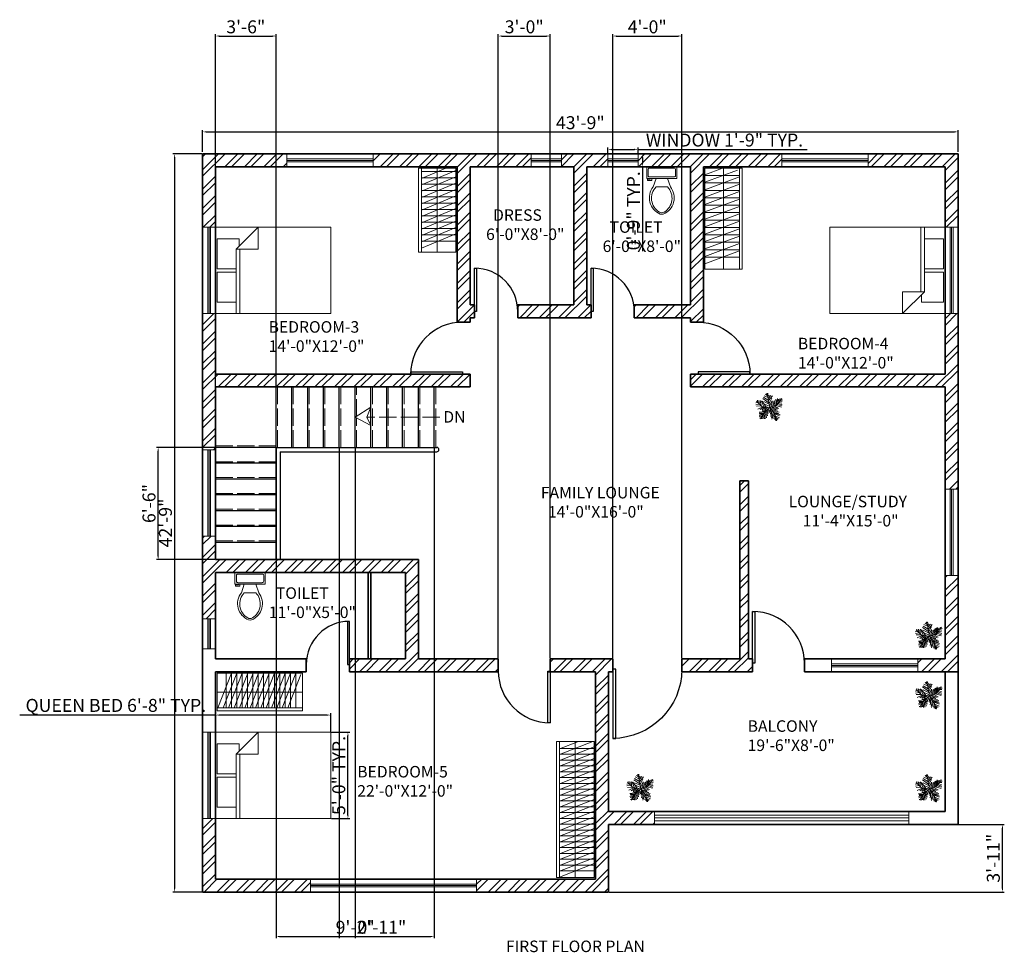
# Model space of a CAD drawing. Units: inches. Extents: x 451 to 1761, y 2292 to 3014.
# Tile 3 of 3: x 1077 to 1761, y 2303 to 2952. Entities that reach past the tile are written whole.
import ezdxf

# ---------------------------------------------------------------- set-up
doc = ezdxf.new("R2010")
doc.units = ezdxf.units.IN
doc.linetypes.add('ACAD_ISO02W100', pattern=[15, 12, -3])
for name, color, linetype, lineweight in [('A-ANNO-DIMS', 2, 'Continuous', 18), ('A-ANNO-PATH', 7, 'ACAD_ISO02W100', 18), ('A-ANNO-SYMB', 7, 'Continuous', 18), ('A-ANNO-TEXT', 7, 'Continuous', 25), ('A-AREA-IDEN', 7, 'Continuous', 18), ('A-DOOR', 4, 'Continuous', 25), ('A-FLOR-CASE', 9, 'Continuous', 18), ('A-FLOR-CASE-PATT', 252, 'Continuous', 13), ('A-FLOR-FIXT', 9, 'Continuous', 18), ('A-FLOR-RAIL', 244, 'Continuous', 18), ('A-FLOR-STRS', 7, 'Continuous', 25), ('A-FLOR-STRS-HIDN', 8, 'ACAD_ISO02W100', 13), ('A-FURN', 8, 'Continuous', 18), ('A-GLAZ', 244, 'Continuous', 18), ('A-WALL', 7, 'Continuous', 35), ('A-WALL-PATT', 252, 'Continuous', 13), ('L-PLNT', 3, 'Continuous', 18)]:
    doc.layers.add(name, color=color, linetype=linetype, lineweight=lineweight)
doc.styles.get("Standard").update_dxf_attribs({"font": 'arial.ttf'})
doc.dimstyles.new('ISO-25', dxfattribs={"dimtxt": 9, "dimasz": 2.5, "dimexe": 1.25, "dimexo": 0.625, "dimtad": 1, "dimlunit": 3, "dimtxsty": 'Standard', "dimcen": 2.5, "dimadec": 0, "dimazin": 0, "dimtfac": 1, "dimtmove": 0, "dimatfit": 3, "dimfxl": 1, "dimarcsym": 0})

# ---------------------------------------------------------------- blocks, each defined once
blk = doc.blocks.new('*U14')
for p, q in [((-40, 0), (-40, 6)), ((0, 0), (0, 6))]:
    blk.add_line(p, q)
blk.add_lwpolyline([(0, 0), (0, -40), (-1.75, -40), (-1.75, 0)], close=True)
blk.add_arc((0, 0), 40, 180, 270)
blk = doc.blocks.new('*U15')
for p, q in [((0, 0), (0, -6)), ((-40, 0), (-40, -6))]:
    blk.add_line(p, q)
blk.add_lwpolyline([(0, 0), (0, 40), (-1.75, 40), (-1.75, 0)], close=True)
blk.add_arc((0, 0), 40, 90, 180)
blk = doc.blocks.new('*U16')
for p, q in [((0, 0), (0, -6)), ((40, 0), (40, -6))]:
    blk.add_line(p, q)
blk.add_lwpolyline([(0, 0), (0, 40), (1.75, 40), (1.75, 0)], close=True)
blk.add_arc((0, 0), 40, 0, 90)
blk = doc.blocks.new('Bed - Queen')
for p, q in [((0, -80.00003), (0, 0)), ((0, 0), (59.99999, 0)), ((59.99999, 0), (59.99999, -80.00003)), ((7.99999, -1.2), (28.79998, -1.2)), ((7.99999, -14.4), (7.99999, -1.2)), ((28.79998, -1.2), (28.79998, -14.4)), ((31.19999, -1.2), (51.99999, -1.2)), ((31.19999, -14.4), (31.19999, -1.2)), ((51.99999, -1.2), (51.99999, -16.4)), ((0, -14.4), (44.8, -14.4)), ((44.8, -16.8), (0, -16.8)), ((59.99999, -29.6), (44.8, -14.4)), ((44.8, -14.4), (44.8, -29.6)), ((51.99999, -16.4), (46.79936, -16.4)), ((44.8, -29.6), (59.99999, -29.6)), ((59.99999, -80.00003), (0, -80.00003))]:
    blk.add_line(p, q)
blk = doc.blocks.new('*U10')
for p, q in [((9.5, -6), (9.5, -2)), ((-10, -8.5), (-8, -8.5)), ((-10, -9.5), (-10, -8.5)), ((-7, -9.5), (-10, -9.5)), ((-8, -8.5), (-8, -8)), ((-7, -8), (-7, -9.5)), ((-4, -8), (-6, -14)), ((4, -8), (6, -14)), ((4, -14), (-4, -14))]:
    blk.add_line(p, q)
blk.add_lwpolyline([(10.5, -8), (10.5, 0), (-10.5, 0), (-10.5, -8)], close=True)
for points in [[(-9.5, -2), (-9.5, -6)], [(8.5, -1), (-8.5, -1)], [(-8.5, -7), (8.5, -7)]]:
    blk.add_lwpolyline(points)
for centre, radius, start, end in [((-8.62, -1.88), 0.884, 81.8699, 188.1301), ((-8.62, -6.12), 0.884, 171.8699, 278.1301), ((8.62, -1.88), 0.884, 351.8699, 98.1301), ((8.62, -6.12), 0.884, 261.8699, 8.1301), ((3.52, -21.58), 12.17, 141.46911, 247.97143), ((4.2, -21.82), 11.33, 136.36773, 238.94682), ((-3.52, -21.58), 12.17, 292.02843, 38.53071), ((-4.2, -21.82), 11.33, 301.05301, 43.63209), ((0, -27.88), 4, 245.73182, 294.26817), ((0, -29), 4, 254.86053, 285.13947)]:
    blk.add_arc(centre, radius, start, end)
blk = doc.blocks.new('*U12')
for p, q in [((-5.114, 28.097), (-24.676, 40.636)), ((-7.288, 39.707), (-21.778, 46.673)), ((-8.737, 47.138), (-17.069, 52.711)), ((-10.186, 53.64), (-13.084, 55.962)), ((0, 0), (-10.5, 57)), ((-9.099, 51.782), (-6.563, 55.962)), ((-7.65, 43.423), (-2.578, 49.46)), ((-5.839, 35.992), (4.667, 48.067)), ((-5.114, 27.632), (10.463, 46.673)), ((-47.498, 19.737), (-55.83, 18.344)), ((-40.615, 13.7), (-55.105, 10.913)), ((-31.5, 4.5), (-52.5, 25.5)), ((-33.37, 6.269), (-52.207, 5.34)), ((-48.585, 21.131), (-49.309, 29.026)), ((-28.299, 3.483), (-47.86, -5.805)), ((-43.513, 28.561), (-42.427, 15.558)), ((-38.442, 26.239), (-34.819, 7.663)), ((-21.416, 3.018), (-38.079, -8.128)), ((-35.544, 28.097), (-24.314, 3.947)), ((0, 0), (-31.5, 4.5)), ((-14.533, 2.09), (-30.834, 25.31)), ((-15.982, 2.09), (-30.11, -9.521)), ((-3.665, 19.273), (-27.574, 35.527)), ((-24.314, 23.917), (-2.941, 13.7)), ((0, 0), (-22.5, -19.5)), ((-6.563, 1.161), (-21.416, -8.128)), ((-20.691, 13.7), (-1.129, 4.876)), ((-2.941, 16.486), (8.652, 37.85)), ((-1.129, 6.734), (9.014, 26.704)), ((0, 0), (27, 9)), ((0, 0), (18, -22.5)), ((3.942, 1.625), (11.187, 24.381)), ((6.478, 1.625), (26.04, -8.592)), ((10.101, 3.483), (17.708, 26.239)), ((11.187, 3.483), (30.749, -5.805)), ((16.259, 5.805), (23.142, 31.348)), ((18.07, 5.805), (35.096, -3.483)), ((22.055, 7.198), (27.489, 32.277)), ((24.229, 7.663), (46.688, 1.625)), ((27, 9), (48, 36)), ((27.127, 9.056), (31.112, 35.992)), ((29.662, 12.307), (48.137, 6.269)), ((31.836, 30.883), (32.561, 16.486)), ((33.285, 16.486), (48.862, 10.913)), ((35.096, 32.741), (37.27, 22.524)), ((36.183, 19.737), (48.137, 17.88)), ((38.719, 34.134), (41.979, 28.561)), ((40.53, 25.775), (48.862, 24.846)), ((43.791, 29.954), (51.036, 30.883)), ((44.153, 36.456), (45.239, 32.741)), ((-17.431, -15.094), (-42.789, -18.809)), ((-28.299, -29.026), (-42.789, -31.348)), ((-24.314, -21.596), (-42.427, -22.06)), ((-30.834, -34.135), (-42.427, -35.528)), ((-26.849, -26.24), (-40.253, -25.775)), ((-22.5, -19.5), (-37.5, -45)), ((-32.646, -36.921), (-31.921, -44.352)), ((-15.257, -12.772), (-30.11, -12.772)), ((-29.023, -30.884), (-27.936, -43.887)), ((-25.038, -23.918), (-22.865, -45.281)), ((-20.691, -18.345), (-17.793, -44.352)), ((-6.563, -5.805), (-19.967, -9.985)), ((-17.069, -15.094), (-12.721, -40.172)), ((-13.446, -11.378), (-8.737, -32.741)), ((-9.461, -8.592), (-6.201, -23.453)), ((-4.752, -3.483), (-3.665, -14.629)), ((2.493, -3.019), (-1.491, -20.202)), ((1.769, -2.555), (24.229, -9.521)), ((5.029, -6.27), (2.131, -25.775)), ((9.014, -11.378), (3.58, -35.992)), ((14.085, -16.951), (6.478, -40.172)), ((7.565, -9.056), (32.198, -14.629)), ((18.07, -22.524), (8.289, -45.745)), ((12.274, -15.094), (36.907, -18.809)), ((20.244, -30.419), (15.897, -44.816)), ((16.259, -19.738), (36.183, -22.989)), ((18, -22.5), (27, -52.5)), ((18.433, -22.524), (40.53, -29.026)), ((19.157, -25.311), (38.719, -33.206)), ((22.78, -37.85), (19.519, -48.532)), ((21.331, -32.741), (39.081, -40.636)), ((22.78, -38.314), (34.372, -44.816)), ((-34.457, -39.708), (-40.978, -42.494)), ((24.591, -45.745), (23.142, -50.854)), ((24.591, -43.423), (30.749, -47.603)), ((26.764, -49.925), (28.213, -50.854))]:
    blk.add_line(p, q)
blk = doc.blocks.new('*D19')
at = {"layer": 'A-ANNO-DIMS', "color": 0, "lineweight": -2, "transparency": 16777216}
for p, q in [((1203.82, 2859.74), (1203.82, 2874.82)), ((1728.82, 2859.74), (1728.82, 2874.82)), ((1206.32, 2873.57), (1726.32, 2873.57))]:
    blk.add_line(p, q, dxfattribs=at)
at = {"layer": 'A-ANNO-DIMS', "color": 0, "transparency": 16777216}
for points in [[(1206.32, 2873.99), (1206.32, 2873.15), (1203.82, 2873.57)], [(1726.32, 2873.99), (1726.32, 2873.15), (1728.82, 2873.57)]]:
    blk.add_solid(points, dxfattribs=at)
at = {"layer": 'Defpoints', "color": 0, "transparency": 16777216}
for p in [(1728.82, 2873.57), (1203.82, 2859.11), (1728.82, 2859.11)]:
    blk.add_point(p, dxfattribs=at)
at = {"layer": 'A-ANNO-DIMS', "color": 0, "transparency": 16777216, "insert": (1466.32, 2878.79), "char_height": 9, "attachment_point": 5}
blk.add_mtext('43\'-9"', dxfattribs=at)
blk = doc.blocks.new('*D20')
at = {"layer": 'A-ANNO-DIMS', "color": 0, "lineweight": -2, "transparency": 16777216}
for p, q in [((1203.19, 2858.28), (1183.1, 2858.28)), ((1184.35, 2855.78), (1184.35, 2347.78)), ((1203.19, 2345.28), (1183.1, 2345.28))]:
    blk.add_line(p, q, dxfattribs=at)
at = {"layer": 'A-ANNO-DIMS', "color": 0, "transparency": 16777216}
for points in [[(1183.94, 2855.78), (1184.77, 2855.78), (1184.35, 2858.28)], [(1183.94, 2347.78), (1184.77, 2347.78), (1184.35, 2345.28)]]:
    blk.add_solid(points, dxfattribs=at)
at = {"layer": 'Defpoints', "color": 0, "transparency": 16777216}
for p in [(1203.82, 2858.28), (1184.35, 2345.28), (1203.82, 2345.28)]:
    blk.add_point(p, dxfattribs=at)
at = {"layer": 'A-ANNO-DIMS', "color": 0, "transparency": 16777216, "insert": (1179.13, 2601.78), "char_height": 9, "attachment_point": 5, "rotation": 90}
blk.add_mtext('42\'-9"', dxfattribs=at)
blk = doc.blocks.new('WIN-60IN')
for p, q in [((0, 5.5), (60, 5.5)), ((0, 4.5), (60, 4.5)), ((0, 3.5), (60, 3.5))]:
    blk.add_line(p, q)
blk.add_lwpolyline([(0, 0), (0, 9), (60, 9), (60, 0)], close=True)
blk = doc.blocks.new('WIN-21IN')
for p, q in [((3.5, 0), (3.5, 21)), ((4.5, 0), (4.5, 21)), ((5.5, 0), (5.5, 21))]:
    blk.add_line(p, q)
blk.add_lwpolyline([(0, 0), (0, 21), (9, 21), (9, 0)], close=True)
blk = doc.blocks.new('*D26')
at = {"layer": 'A-ANNO-DIMS', "color": 0, "lineweight": -2, "transparency": 16777216}
for p, q in [((1212.82, 2468.28), (1076.68, 2468.28)), ((1212.82, 2456.9), (1212.82, 2469.53)), ((1290.32, 2468.28), (1215.32, 2468.28)), ((1292.82, 2456.9), (1292.82, 2469.53))]:
    blk.add_line(p, q, dxfattribs=at)
at = {"layer": 'A-ANNO-DIMS', "color": 0, "transparency": 16777216}
for points in [[(1215.32, 2468.69), (1215.32, 2467.86), (1212.82, 2468.28)], [(1290.32, 2468.69), (1290.32, 2467.86), (1292.82, 2468.28)]]:
    blk.add_solid(points, dxfattribs=at)
at = {"layer": 'Defpoints', "color": 0, "transparency": 16777216}
for p in [(1212.82, 2468.28), (1212.82, 2456.28), (1292.82, 2456.28)]:
    blk.add_point(p, dxfattribs=at)
at = {"layer": 'A-ANNO-DIMS', "color": 0, "transparency": 16777216, "insert": (1143.5, 2473.83), "char_height": 9, "attachment_point": 5}
blk.add_mtext('QUEEN BED 6\'-8" TYP.', dxfattribs=at)
blk = doc.blocks.new('*D27')
at = {"layer": 'A-ANNO-DIMS', "color": 0, "lineweight": -2, "transparency": 16777216}
for p, q in [((1293.44, 2456.28), (1306.07, 2456.28)), ((1304.82, 2398.78), (1304.82, 2453.78)), ((1293.44, 2396.28), (1306.07, 2396.28))]:
    blk.add_line(p, q, dxfattribs=at)
at = {"layer": 'A-ANNO-DIMS', "color": 0, "transparency": 16777216}
for points in [[(1304.4, 2453.78), (1305.23, 2453.78), (1304.82, 2456.28)], [(1304.4, 2398.78), (1305.23, 2398.78), (1304.82, 2396.28)]]:
    blk.add_solid(points, dxfattribs=at)
at = {"layer": 'Defpoints', "color": 0, "transparency": 16777216}
for p in [(1292.82, 2456.28), (1304.82, 2456.28), (1292.82, 2396.28)]:
    blk.add_point(p, dxfattribs=at)
at = {"layer": 'A-ANNO-DIMS', "color": 0, "transparency": 16777216, "insert": (1299.6, 2426.28), "char_height": 9, "attachment_point": 5, "rotation": 90}
blk.add_mtext('5\'-0" TYP.', dxfattribs=at)
blk = doc.blocks.new('*D28')
at = {"layer": 'A-ANNO-DIMS', "color": 0, "lineweight": -2, "transparency": 16777216}
for p, q in [((1485.42, 2858.9), (1485.42, 2862.68)), ((1487.92, 2861.43), (1503.92, 2861.43)), ((1506.42, 2858.9), (1506.42, 2862.68)), ((1506.42, 2861.43), (1624.06, 2861.43))]:
    blk.add_line(p, q, dxfattribs=at)
at = {"layer": 'A-ANNO-DIMS', "color": 0, "transparency": 16777216}
for points in [[(1487.92, 2861.84), (1487.92, 2861.01), (1485.42, 2861.43)], [(1503.92, 2861.84), (1503.92, 2861.01), (1506.42, 2861.43)]]:
    blk.add_solid(points, dxfattribs=at)
at = {"layer": 'Defpoints', "color": 0, "transparency": 16777216}
for p in [(1506.42, 2861.43), (1485.42, 2858.28), (1506.42, 2858.28)]:
    blk.add_point(p, dxfattribs=at)
at = {"layer": 'A-ANNO-DIMS', "color": 0, "transparency": 16777216, "insert": (1566.49, 2866.71), "char_height": 9, "attachment_point": 5}
blk.add_mtext('WINDOW 1\'-9" TYP.', dxfattribs=at)
blk = doc.blocks.new('*D29')
at = {"layer": 'A-ANNO-DIMS', "color": 0, "lineweight": -2, "transparency": 16777216}
for p, q in [((1507.05, 2858.28), (1510.82, 2858.28)), ((1509.57, 2855.78), (1509.57, 2851.78)), ((1507.05, 2849.28), (1510.82, 2849.28)), ((1509.57, 2849.28), (1509.57, 2790.67))]:
    blk.add_line(p, q, dxfattribs=at)
at = {"layer": 'A-ANNO-DIMS', "color": 0, "transparency": 16777216}
for points in [[(1509.16, 2855.78), (1509.99, 2855.78), (1509.57, 2858.28)], [(1509.16, 2851.78), (1509.99, 2851.78), (1509.57, 2849.28)]]:
    blk.add_solid(points, dxfattribs=at)
at = {"layer": 'Defpoints', "color": 0, "transparency": 16777216}
for p in [(1506.42, 2858.28), (1506.42, 2849.28), (1509.57, 2849.28)]:
    blk.add_point(p, dxfattribs=at)
at = {"layer": 'A-ANNO-DIMS', "color": 0, "transparency": 16777216, "insert": (1504.35, 2818.72), "char_height": 9, "attachment_point": 5, "rotation": 90}
blk.add_mtext('0\'-9" TYP.', dxfattribs=at)
blk = doc.blocks.new('*D41')
at = {"layer": 'A-ANNO-DIMS', "color": 0, "lineweight": -2, "transparency": 16777216}
for p, q in [((1254.82, 2653.65), (1254.82, 2313.13)), ((1364.82, 2653.65), (1364.82, 2313.13)), ((1257.32, 2314.38), (1362.32, 2314.38))]:
    blk.add_line(p, q, dxfattribs=at)
at = {"layer": 'A-ANNO-DIMS', "color": 0, "transparency": 16777216}
for points in [[(1257.32, 2314.79), (1257.32, 2313.96), (1254.82, 2314.38)], [(1362.32, 2314.79), (1362.32, 2313.96), (1364.82, 2314.38)]]:
    blk.add_solid(points, dxfattribs=at)
at = {"layer": 'Defpoints', "color": 0, "transparency": 16777216}
for p in [(1254.82, 2654.28), (1364.82, 2654.28), (1364.82, 2314.38)]:
    blk.add_point(p, dxfattribs=at)
at = {"layer": 'A-ANNO-DIMS', "color": 0, "transparency": 16777216, "insert": (1309.82, 2319.6), "char_height": 9, "attachment_point": 5}
blk.add_mtext('9\'-2"', dxfattribs=at)
blk = doc.blocks.new('*D42')
at = {"layer": 'A-ANNO-DIMS', "color": 0, "lineweight": -2, "transparency": 16777216}
for p, q in [((1212.19, 2654.28), (1171.67, 2654.28)), ((1172.92, 2578.78), (1172.92, 2651.78)), ((1212.19, 2576.28), (1171.67, 2576.28))]:
    blk.add_line(p, q, dxfattribs=at)
at = {"layer": 'A-ANNO-DIMS', "color": 0, "transparency": 16777216}
for points in [[(1172.5, 2651.78), (1173.33, 2651.78), (1172.92, 2654.28)], [(1172.5, 2578.78), (1173.33, 2578.78), (1172.92, 2576.28)]]:
    blk.add_solid(points, dxfattribs=at)
at = {"layer": 'Defpoints', "color": 0, "transparency": 16777216}
for p in [(1172.92, 2654.28), (1212.82, 2654.28), (1212.82, 2576.28)]:
    blk.add_point(p, dxfattribs=at)
at = {"layer": 'A-ANNO-DIMS', "color": 0, "transparency": 16777216, "insert": (1167.7, 2615.28), "char_height": 9, "attachment_point": 5, "rotation": 90}
blk.add_mtext('6\'-6"', dxfattribs=at)
blk = doc.blocks.new('*D43')
at = {"layer": 'A-ANNO-DIMS', "color": 0, "lineweight": -2, "transparency": 16777216}
for p, q in [((1212.82, 2576.9), (1212.82, 2941.43)), ((1215.32, 2940.18), (1252.32, 2940.18)), ((1254.82, 2576.9), (1254.82, 2941.43))]:
    blk.add_line(p, q, dxfattribs=at)
at = {"layer": 'A-ANNO-DIMS', "color": 0, "transparency": 16777216}
for points in [[(1215.32, 2940.59), (1215.32, 2939.76), (1212.82, 2940.18)], [(1252.32, 2940.59), (1252.32, 2939.76), (1254.82, 2940.18)]]:
    blk.add_solid(points, dxfattribs=at)
at = {"layer": 'Defpoints', "color": 0, "transparency": 16777216}
for p in [(1254.82, 2940.18), (1212.82, 2576.28), (1254.82, 2576.28)]:
    blk.add_point(p, dxfattribs=at)
at = {"layer": 'A-ANNO-DIMS', "color": 0, "transparency": 16777216, "insert": (1233.82, 2945.4), "char_height": 9, "attachment_point": 5}
blk.add_mtext('3\'-6"', dxfattribs=at)
blk = doc.blocks.new('*D44')
at = {"layer": 'A-ANNO-DIMS', "color": 0, "lineweight": -2, "transparency": 16777216}
for p, q in [((1298.82, 2653.65), (1298.82, 2313.13)), ((1309.82, 2653.65), (1309.82, 2313.13)), ((1301.32, 2314.38), (1307.32, 2314.38)), ((1309.82, 2314.38), (1344.48, 2314.38))]:
    blk.add_line(p, q, dxfattribs=at)
at = {"layer": 'A-ANNO-DIMS', "color": 0, "transparency": 16777216}
for points in [[(1301.32, 2314.79), (1301.32, 2313.96), (1298.82, 2314.38)], [(1307.32, 2314.79), (1307.32, 2313.96), (1309.82, 2314.38)]]:
    blk.add_solid(points, dxfattribs=at)
at = {"layer": 'Defpoints', "color": 0, "transparency": 16777216}
for p in [(1298.82, 2654.28), (1309.82, 2654.28), (1309.82, 2314.38)]:
    blk.add_point(p, dxfattribs=at)
at = {"layer": 'A-ANNO-DIMS', "color": 0, "transparency": 16777216, "insert": (1328.4, 2319.6), "char_height": 9, "attachment_point": 5}
blk.add_mtext('0\'-11"', dxfattribs=at)
blk = doc.blocks.new('*D45')
at = {"layer": 'A-ANNO-DIMS', "color": 0, "lineweight": -2, "transparency": 16777216}
for p, q in [((1486.44, 2392.24), (1760.97, 2392.24)), ((1759.72, 2347.78), (1759.72, 2389.74)), ((1486.44, 2345.28), (1760.97, 2345.28))]:
    blk.add_line(p, q, dxfattribs=at)
at = {"layer": 'A-ANNO-DIMS', "color": 0, "transparency": 16777216}
for points in [[(1759.3, 2389.74), (1760.13, 2389.74), (1759.72, 2392.24)], [(1759.3, 2347.78), (1760.13, 2347.78), (1759.72, 2345.28)]]:
    blk.add_solid(points, dxfattribs=at)
at = {"layer": 'Defpoints', "color": 0, "transparency": 16777216}
for p in [(1485.82, 2392.24), (1759.72, 2392.24), (1485.82, 2345.28)]:
    blk.add_point(p, dxfattribs=at)
at = {"layer": 'A-ANNO-DIMS', "color": 0, "transparency": 16777216, "insert": (1754.49, 2368.76), "char_height": 9, "attachment_point": 5, "rotation": 90}
blk.add_mtext('3\'-11"', dxfattribs=at)
blk = doc.blocks.new('*D46')
at = {"layer": 'A-ANNO-DIMS', "color": 0, "lineweight": -2, "transparency": 16777216}
for p, q in [((1409.32, 2507.9), (1409.32, 2941.43)), ((1411.82, 2940.18), (1442.82, 2940.18)), ((1445.32, 2507.9), (1445.32, 2941.43))]:
    blk.add_line(p, q, dxfattribs=at)
at = {"layer": 'A-ANNO-DIMS', "color": 0, "transparency": 16777216}
for points in [[(1411.82, 2940.59), (1411.82, 2939.76), (1409.32, 2940.18)], [(1442.82, 2940.59), (1442.82, 2939.76), (1445.32, 2940.18)]]:
    blk.add_solid(points, dxfattribs=at)
at = {"layer": 'Defpoints', "color": 0, "transparency": 16777216}
for p in [(1445.32, 2940.18), (1409.32, 2507.28), (1445.32, 2507.28)]:
    blk.add_point(p, dxfattribs=at)
at = {"layer": 'A-ANNO-DIMS', "color": 0, "transparency": 16777216, "insert": (1427.32, 2945.4), "char_height": 9, "attachment_point": 5}
blk.add_mtext('3\'-0"', dxfattribs=at)
blk = doc.blocks.new('*D47')
at = {"layer": 'A-ANNO-DIMS', "color": 0, "lineweight": -2, "transparency": 16777216}
for p, q in [((1488.82, 2507.9), (1488.82, 2941.43)), ((1491.32, 2940.18), (1534.32, 2940.18)), ((1536.82, 2507.9), (1536.82, 2941.43))]:
    blk.add_line(p, q, dxfattribs=at)
at = {"layer": 'A-ANNO-DIMS', "color": 0, "transparency": 16777216}
for points in [[(1491.32, 2940.59), (1491.32, 2939.76), (1488.82, 2940.18)], [(1534.32, 2940.59), (1534.32, 2939.76), (1536.82, 2940.18)]]:
    blk.add_solid(points, dxfattribs=at)
at = {"layer": 'Defpoints', "color": 0, "transparency": 16777216}
for p in [(1536.82, 2940.18), (1488.82, 2507.28), (1536.82, 2507.28)]:
    blk.add_point(p, dxfattribs=at)
at = {"layer": 'A-ANNO-DIMS', "color": 0, "transparency": 16777216, "insert": (1512.82, 2945.4), "char_height": 9, "attachment_point": 5}
blk.add_mtext('4\'-0"', dxfattribs=at)

msp = doc.modelspace()

# ---------------------------------------------------------------- hatches: boundary and pattern name
at = {"layer": 'A-FLOR-CASE-PATT'}
h = msp.add_hatch(dxfattribs=at)
h.set_pattern_fill('ANSI31', color=256, scale=1.281376, angle=-22.43333, style=0)
h.paths.add_polyline_path([(1355.816, 2789.86), (1379.816, 2799.834), (1379.816, 2848.297), (1369.164, 2848.276), (1355.816, 2842.729)])
h = msp.add_hatch(dxfattribs=at)
h.set_pattern_fill('ANSI31', color=256, scale=1.387624, angle=-45, style=0)
h.paths.add_polyline_path([(1355.816, 2794.266), (1379.816, 2794.266), (1379.816, 2847.135), (1355.816, 2847.135)])
h = msp.add_hatch(dxfattribs=at)
h.set_pattern_fill('ANSI31', color=256, scale=1.520558, angle=-24.6033, style=0)
h.paths.add_polyline_path([(1552.816, 2778.252), (1576.816, 2787.176), (1576.816, 2843.834), (1574.909, 2848.276), (1561.057, 2848.276), (1552.816, 2845.212)])
h = msp.add_hatch(dxfattribs=at)
h.set_pattern_fill('ANSI31', color=256, scale=1.622274, angle=135, style=0)
h.paths.add_polyline_path([(1552.816, 2783.403), (1576.816, 2783.403), (1576.816, 2845.212), (1552.816, 2845.212)])
h = msp.add_hatch(dxfattribs=at)
h.set_pattern_fill('ANSI31', color=256, scale=1.0926, angle=23.3975, style=0)
h.paths.add_polyline_path([(1213.816, 2473.276), (1266.051, 2473.276), (1273.315, 2491.62), (1271.824, 2497.276), (1223.319, 2497.276)])
h = msp.add_hatch(dxfattribs=at)
h.set_pattern_fill('ANSI31', color=256, scale=1.175145, angle=45, style=0)
h.paths.add_polyline_path([(1217.547, 2473.276), (1269.782, 2473.276), (1269.782, 2497.276), (1217.547, 2497.276)])
h = msp.add_hatch(dxfattribs=at)
h.set_pattern_fill('ANSI31', color=256, scale=1.188375, angle=-23.51425, style=0)
h.paths.add_polyline_path([(1451.816, 2355.276), (1475.816, 2364.723), (1475.816, 2449.875), (1465.831, 2450), (1455.529, 2450), (1451.816, 2448.538)])
h = msp.add_hatch(dxfattribs=at)
h.set_pattern_fill('ANSI31', color=256, scale=1.277126, angle=-45, style=0)
h.paths.add_polyline_path([(1451.816, 2359.331), (1475.816, 2359.331), (1475.816, 2448.538), (1451.816, 2448.538)])
at = {"layer": 'A-WALL-PATT'}
h = msp.add_hatch(dxfattribs=at)
h.set_pattern_fill('ANSI32', color=256)
h.paths.add_polyline_path([(1473.81, 2753.276), (1470.816, 2753.276), (1470.816, 2849.276), (1485.423, 2849.276), (1485.423, 2858.276), (1453.123, 2858.276), (1453.123, 2849.276), (1461.816, 2849.276), (1461.816, 2753.276), (1422.483, 2753.276, -0.0376447), (1422.822, 2748.777), (1422.822, 2744.276), (1473.81, 2744.276), (1473.81, 2748.777)])
h.paths.add_polyline_path([(1551.816, 2849.276), (1606.235, 2849.276), (1606.235, 2858.276), (1506.423, 2858.276), (1506.423, 2849.276), (1542.816, 2849.276), (1542.816, 2753.276), (1503.816, 2753.276), (1503.816, 2744.276), (1542.816, 2744.276), (1542.816, 2741.276), (1548.216, 2741.276), (1551.816, 2741.276)])
h.paths.add_polyline_path([(1392.816, 2753.276), (1389.816, 2753.276), (1389.816, 2849.276), (1432.123, 2849.276), (1432.123, 2858.276), (1380.816, 2858.276), (1322.316, 2858.276), (1322.316, 2849.276), (1380.816, 2849.276), (1380.816, 2741.276), (1389.816, 2741.276), (1389.816, 2744.276), (1392.816, 2744.276)])
h.paths.add_polyline_path([(1728.816, 2747.276), (1719.816, 2747.276), (1719.816, 2705.276), (1551.816, 2705.276), (1548.216, 2705.276), (1542.816, 2705.276), (1542.816, 2696.276), (1719.816, 2696.276), (1719.816, 2625.296), (1728.816, 2625.296)])
h.paths.add_polyline_path([(1212.816, 2849.276), (1262.316, 2849.276), (1262.316, 2858.276), (1203.816, 2858.276), (1203.816, 2807.276), (1212.816, 2807.276)])
h.paths.add_polyline_path([(1728.816, 2858.276), (1666.235, 2858.276), (1666.235, 2849.276), (1719.816, 2849.276), (1719.816, 2807.276), (1728.816, 2807.276)])
h.paths.add_polyline_path([(1353.816, 2576.276), (1212.816, 2576.276), (1212.816, 2592.62), (1203.816, 2592.62), (1203.816, 2535.234), (1212.816, 2535.234), (1212.816, 2567.276), (1344.816, 2567.276), (1344.816, 2507.276), (1305.816, 2507.276), (1305.816, 2503.377), (1305.816, 2498.276), (1409.316, 2498.276), (1409.316, 2507.276), (1353.816, 2507.276)])
h.paths.add_polyline_path([(1728.816, 2565.296), (1719.816, 2565.296), (1719.816, 2507.276), (1700.944, 2507.276), (1700.944, 2498.276), (1719.816, 2498.276), (1728.816, 2498.276)])
h.paths.add_polyline_path([(1583.073, 2631.034), (1577.073, 2631.034), (1577.073, 2507.276), (1536.816, 2507.276), (1536.816, 2498.276), (1586.073, 2498.276), (1586.073, 2507.276), (1583.073, 2507.276)])
h = msp.add_hatch(dxfattribs=at)
h.set_pattern_fill('ANSI32', color=256)
h.paths.add_polyline_path([(1389.816, 2705.276), (1384.416, 2705.276), (1348.416, 2705.276), (1212.816, 2705.276), (1212.816, 2747.276), (1203.816, 2747.276), (1203.816, 2652.62), (1212.816, 2652.62), (1212.816, 2696.276), (1389.816, 2696.276)])
h.paths.add_polyline_path([(1278.816, 2354.276), (1212.816, 2354.276), (1212.816, 2396.276), (1203.816, 2396.276), (1203.816, 2345.276), (1278.816, 2345.276)])
h = msp.add_hatch(dxfattribs=at)
h.set_pattern_fill('ANSI32', color=256)
h.paths.add_polyline_path([(1485.816, 2392.237), (1517.902, 2392.237), (1517.902, 2401.237), (1485.816, 2401.237), (1485.816, 2498.276), (1488.816, 2498.276), (1488.816, 2507.276), (1445.316, 2507.276), (1445.316, 2498.276), (1476.816, 2498.276), (1476.816, 2354.276), (1394.234, 2354.276), (1394.234, 2345.276), (1485.816, 2345.276)])

# ---------------------------------------------------------------- linework, layer by layer
at = {"layer": 'A-ANNO-PATH'}
msp.add_line((1368.565, 2675.276), (1317.944, 2675.276), dxfattribs=at)
at = {"layer": 'A-ANNO-SYMB'}
for p, q in [((1309.816, 2675.276), (1320.816, 2682.17)), ((1317.944, 2675.276), (1320.816, 2682.17)), ((1309.816, 2675.276), (1320.816, 2669.469)), ((1320.816, 2669.469), (1317.944, 2675.276))]:
    msp.add_line(p, q, dxfattribs=at)
at = {"layer": 'A-FLOR-CASE'}
for p, q in [((1353.816, 2848.276), (1379.816, 2848.276)), ((1353.816, 2848.276), (1353.816, 2789.86)), ((1355.816, 2848.276), (1355.816, 2789.86)), ((1366.816, 2848.276), (1366.816, 2789.86)), ((1379.816, 2848.276), (1379.816, 2789.86)), ((1552.816, 2848.276), (1552.816, 2778.252)), ((1552.816, 2848.276), (1578.816, 2848.276)), ((1565.816, 2848.276), (1565.816, 2778.252)), ((1576.816, 2848.276), (1576.816, 2778.252)), ((1578.816, 2848.276), (1578.816, 2778.252)), ((1379.816, 2789.86), (1353.816, 2789.86)), ((1552.816, 2778.252), (1578.816, 2778.252)), ((1213.816, 2497.276), (1273.315, 2497.276)), ((1213.816, 2497.276), (1213.816, 2471.276)), ((1273.315, 2497.276), (1273.315, 2471.276)), ((1213.816, 2484.276), (1273.315, 2484.276)), ((1213.816, 2473.276), (1273.315, 2473.276)), ((1213.816, 2471.276), (1273.315, 2471.276)), ((1475.816, 2450), (1449.816, 2450)), ((1449.816, 2450), (1449.816, 2355.276)), ((1451.816, 2450), (1451.816, 2355.276)), ((1462.816, 2355.276), (1462.816, 2450)), ((1475.816, 2450), (1475.816, 2355.276)), ((1449.816, 2355.276), (1475.816, 2355.276))]:
    msp.add_line(p, q, dxfattribs=at)
at = {"layer": 'A-FLOR-RAIL'}
for p, q in [((1517.902, 2392.237), (1517.902, 2401.237)), ((1517.902, 2398.737), (1694.603, 2398.737)), ((1517.902, 2396.737), (1694.603, 2396.737)), ((1694.603, 2401.237), (1694.603, 2392.237)), ((1517.902, 2394.737), (1694.603, 2394.737))]:
    msp.add_line(p, q, dxfattribs=at)
at = {"layer": 'A-FLOR-STRS'}
for p, q in [((1254.816, 2654.276), (1254.816, 2696.276)), ((1265.816, 2654.276), (1265.816, 2696.276)), ((1276.816, 2654.276), (1276.816, 2696.276)), ((1287.816, 2654.276), (1287.816, 2696.276)), ((1298.816, 2654.276), (1298.816, 2696.276)), ((1309.816, 2654.276), (1309.816, 2696.276)), ((1320.816, 2654.276), (1320.816, 2696.276)), ((1331.816, 2654.276), (1331.816, 2696.276)), ((1342.816, 2654.276), (1342.816, 2696.276)), ((1353.816, 2654.276), (1353.816, 2696.276)), ((1364.816, 2654.276), (1364.816, 2696.276)), ((1254.816, 2654.276), (1212.816, 2654.276)), ((1254.816, 2654.276), (1366.639, 2654.276)), ((1254.816, 2654.276), (1254.816, 2576.276)), ((1257.816, 2651.276), (1366.611, 2651.276)), ((1257.816, 2651.276), (1257.816, 2576.276)), ((1254.816, 2643.276), (1212.816, 2643.276)), ((1254.816, 2632.276), (1212.816, 2632.276)), ((1254.816, 2621.276), (1212.816, 2621.276)), ((1254.816, 2610.276), (1212.816, 2610.276)), ((1254.816, 2599.276), (1212.816, 2599.276)), ((1254.816, 2588.276), (1212.816, 2588.276))]:
    msp.add_line(p, q, dxfattribs=at)
msp.add_arc((1366.468, 2652.777), 1.508, 275.43459, 83.475751, dxfattribs=at)
at = {"layer": 'A-FLOR-STRS-HIDN'}
for p, q in [((1255.816, 2654.276), (1255.816, 2696.276)), ((1266.816, 2654.276), (1266.816, 2696.276)), ((1277.816, 2654.276), (1277.816, 2696.276)), ((1288.816, 2654.276), (1288.816, 2696.276)), ((1299.816, 2654.276), (1299.816, 2696.276)), ((1310.816, 2675.903), (1310.816, 2696.276)), ((1321.816, 2654.276), (1321.816, 2696.276)), ((1332.816, 2654.276), (1332.816, 2696.276)), ((1343.816, 2654.276), (1343.816, 2696.276)), ((1354.816, 2654.276), (1354.816, 2696.276)), ((1365.816, 2654.276), (1365.816, 2696.276)), ((1310.816, 2654.276), (1310.816, 2674.748)), ((1254.816, 2655.276), (1212.816, 2655.276)), ((1254.816, 2644.276), (1212.816, 2644.276)), ((1254.816, 2633.276), (1212.816, 2633.276)), ((1254.816, 2622.276), (1212.816, 2622.276)), ((1254.816, 2611.276), (1212.816, 2611.276)), ((1254.816, 2600.276), (1212.816, 2600.276)), ((1254.816, 2589.276), (1212.816, 2589.276))]:
    msp.add_line(p, q, dxfattribs=at)
at = {"layer": 'A-GLAZ'}
for p, q in [((1278.816, 2350.776), (1394.234, 2350.776)), ((1278.816, 2349.776), (1394.234, 2349.776)), ((1278.816, 2348.776), (1394.234, 2348.776))]:
    msp.add_line(p, q, dxfattribs=at)
msp.add_lwpolyline([(1278.816, 2345.276), (1278.816, 2354.276), (1394.234, 2354.276), (1394.234, 2345.276)], close=True, dxfattribs=at)
at = {"layer": 'A-WALL'}
for p, q in [((1203.816, 2858.276), (1203.816, 2345.276)), ((1203.816, 2858.276), (1380.816, 2858.276)), ((1380.816, 2858.276), (1728.816, 2858.276)), ((1728.816, 2858.276), (1728.816, 2392.237)), ((1212.816, 2849.276), (1212.816, 2705.276)), ((1212.816, 2849.276), (1380.816, 2849.276)), ((1380.816, 2849.276), (1380.816, 2741.276)), ((1389.816, 2849.276), (1389.816, 2753.276)), ((1389.816, 2849.276), (1461.816, 2849.276)), ((1461.816, 2849.276), (1461.816, 2753.276)), ((1470.816, 2849.276), (1470.816, 2753.276)), ((1470.816, 2849.276), (1542.816, 2849.276)), ((1542.816, 2849.276), (1542.816, 2753.276)), ((1551.816, 2849.276), (1551.816, 2741.276)), ((1551.816, 2849.276), (1719.816, 2849.276)), ((1719.816, 2849.276), (1719.816, 2705.276)), ((1389.816, 2753.276), (1392.816, 2753.276)), ((1392.816, 2744.276), (1392.816, 2753.276)), ((1422.816, 2744.276), (1422.816, 2753.276)), ((1422.816, 2753.276), (1461.816, 2753.276)), ((1470.816, 2753.276), (1473.816, 2753.276)), ((1473.816, 2753.276), (1473.816, 2744.276)), ((1503.816, 2753.276), (1503.816, 2744.276)), ((1503.816, 2753.276), (1542.816, 2753.276)), ((1389.816, 2744.276), (1392.816, 2744.276)), ((1389.816, 2744.276), (1389.816, 2741.276)), ((1422.816, 2744.276), (1473.81, 2744.276)), ((1473.81, 2744.276), (1473.816, 2744.276)), ((1503.816, 2744.276), (1542.816, 2744.276)), ((1542.816, 2744.276), (1542.816, 2741.276)), ((1389.816, 2741.276), (1380.816, 2741.276)), ((1542.816, 2741.276), (1551.816, 2741.276)), ((1212.816, 2705.276), (1380.816, 2705.276)), ((1389.816, 2705.276), (1380.816, 2705.276)), ((1389.816, 2705.276), (1389.816, 2696.276)), ((1542.816, 2705.276), (1551.816, 2705.276)), ((1542.816, 2705.276), (1542.816, 2696.276)), ((1551.816, 2705.276), (1719.816, 2705.276)), ((1212.816, 2696.276), (1389.816, 2696.276)), ((1212.816, 2696.276), (1212.816, 2576.276)), ((1542.816, 2696.276), (1719.816, 2696.276)), ((1719.816, 2696.276), (1719.816, 2507.276)), ((1577.073, 2631.034), (1577.073, 2507.276)), ((1577.073, 2631.034), (1583.073, 2631.034)), ((1583.073, 2631.034), (1583.073, 2507.276)), ((1212.816, 2576.276), (1353.816, 2576.276)), ((1353.816, 2576.276), (1353.816, 2507.276)), ((1212.816, 2567.276), (1344.816, 2567.276)), ((1212.816, 2567.276), (1212.816, 2507.276)), ((1318.816, 2567.276), (1318.816, 2507.276)), ((1320.816, 2567.276), (1320.816, 2507.276)), ((1344.816, 2567.276), (1344.816, 2507.276)), ((1212.816, 2507.276), (1275.816, 2507.276)), ((1275.816, 2507.276), (1275.816, 2498.276)), ((1305.816, 2507.276), (1344.816, 2507.276)), ((1305.816, 2507.276), (1305.816, 2498.276)), ((1353.816, 2507.276), (1409.316, 2507.276)), ((1409.316, 2498.276), (1409.316, 2507.276)), ((1445.316, 2498.276), (1445.316, 2507.276)), ((1445.316, 2507.276), (1488.816, 2507.276)), ((1488.816, 2498.276), (1488.816, 2507.276)), ((1536.816, 2507.276), (1577.073, 2507.276)), ((1536.816, 2498.276), (1536.816, 2507.276)), ((1583.073, 2507.276), (1586.073, 2507.276)), ((1586.073, 2507.276), (1586.073, 2498.276)), ((1622.073, 2507.276), (1622.073, 2498.276)), ((1622.073, 2507.276), (1719.816, 2507.276)), ((1212.816, 2498.276), (1275.816, 2498.276)), ((1212.816, 2498.276), (1212.816, 2354.276)), ((1305.816, 2498.276), (1409.316, 2498.276)), ((1409.316, 2498.276), (1409.321, 2498.276)), ((1443.741, 2498.276), (1476.816, 2498.276)), ((1476.816, 2498.276), (1476.816, 2354.276)), ((1485.816, 2498.276), (1485.816, 2401.237)), ((1485.816, 2498.276), (1488.816, 2498.276)), ((1536.816, 2498.276), (1586.073, 2498.276)), ((1622.073, 2498.276), (1719.816, 2498.276)), ((1719.816, 2498.276), (1719.816, 2401.237)), ((1719.816, 2498.276), (1728.816, 2498.276)), ((1485.816, 2401.237), (1719.816, 2401.237)), ((1485.816, 2392.237), (1728.816, 2392.237)), ((1485.816, 2392.237), (1485.816, 2345.276)), ((1212.816, 2354.276), (1476.816, 2354.276)), ((1203.816, 2345.276), (1485.816, 2345.276))]:
    msp.add_line(p, q, dxfattribs=at)

# ---------------------------------------------------------------- block references
at = {"layer": 'A-DOOR'}
for name, p, xscale, yscale, zscale in [('*U16', (1392.816, 2748.777), 0.7501499850030064, 0.7501499850030064, 0.7501499850030064), ('*U16', (1473.81, 2748.777), 0.7501499850030064, 0.7501499850030064, 0.7501499850030064), ('*U16', (1586.073, 2504.276), 0.9, 0.9, 0.9), ('*U15', (1305.816, 2503.377), 0.7501499850030064, 0.7501499850030064, 0.7501499850030064), ('*U14', (1488.807, 2500.076), -1.200000000000005, 1.200000000000005, 1.200000000000005), ('*U14', (1445.316, 2498.876), 0.9, 0.9, 0.9)]:
    msp.add_blockref(name, p, dxfattribs=dict(at, xscale=xscale, yscale=yscale, zscale=zscale))
at = {"layer": 'A-DOOR', "yscale": 0.9, "zscale": 0.9}
for p, xscale, rotation in [((1384.416, 2705.276), 0.9, 270.0000000000043), ((1548.216, 2705.276), -0.9, 89.99999999999568)]:
    msp.add_blockref('*U14', p, dxfattribs=dict(at, xscale=xscale, rotation=rotation))
at = {"layer": 'A-FLOR-FIXT'}
for p in [(1522.915, 2849.276), (1236.761, 2567.276)]:
    msp.add_blockref('*U10', p, dxfattribs=at)
at = {"layer": 'A-FURN'}
for p, rotation in [((1212.816, 2747.276), 90), ((1719.816, 2807.276), 270), ((1212.816, 2396.276), 90)]:
    msp.add_blockref('Bed - Queen', p, dxfattribs=dict(at, rotation=rotation))
at = {"layer": 'A-GLAZ'}
for p in [(1262.316, 2849.276), (1606.235, 2849.276), (1640.944, 2498.276)]:
    msp.add_blockref('WIN-60IN', p, dxfattribs=at)
for name, p, rotation in [('WIN-21IN', (1432.123, 2858.276), 270.0000000000006), ('WIN-21IN', (1485.423, 2858.276), 270.0000000000006), ('WIN-60IN', (1203.816, 2807.276), 270.0000000000009), ('WIN-60IN', (1719.816, 2807.276), 269.9999999999994), ('WIN-60IN', (1203.816, 2652.62), 270.0000000000008), ('WIN-60IN', (1719.816, 2625.296), 270.0000000000003), ('WIN-21IN', (1212.816, 2535.234), 180), ('WIN-60IN', (1203.816, 2456.276), 269.9999999999994)]:
    msp.add_blockref(name, p, dxfattribs=dict(at, rotation=rotation))
at = {"layer": 'L-PLNT', "xscale": 0.1751800968654594, "yscale": 0.1751800968654594, "zscale": 0.1751800968654594}
for p in [(1597.987, 2681.973), (1708.894, 2522.991), (1708.894, 2481.57), (1508.308, 2417.093), (1708.894, 2416.951)]:
    msp.add_blockref('*U12', p, dxfattribs=at)

# ---------------------------------------------------------------- texts
at = {"layer": 'A-ANNO-TEXT', "char_height": 8, "attachment_point": 1}
for s, width, insert in [('DN', 18.28891, (1371.098, 2679.514)), ('FIRST FLOOR PLAN', 109.06769, (1414.593, 2311.53))]:
    msp.add_mtext_dynamic_manual_height_columns(s, width=width, gutter_width=12.5, heights=[0], dxfattribs=dict(at, insert=insert))
at = {"layer": 'A-AREA-IDEN', "char_height": 8, "attachment_point": 1}
for s, width, insert in [('  DRESS \\P6\'-0"X8\'-0"', 53.88421, (1400.801, 2819.758)), ('  TOILET \\P6\'-0"X8\'-0"', 53.88421, (1481.801, 2811.417)), ('BEDROOM-3 \\P14\'-0"X12\'-0"', 68.82431, (1249.685, 2742.02)), ('BEDROOM-4 \\P14\'-0"X12\'-0"', 68.82431, (1617.519, 2730.444)), ('FAMILY LOUNGE \\P  14\'-0"X16\'-0"', 90.64336, (1438.882, 2626.855)), ('LOUNGE/STUDY \\P    11\'-4"X15\'-0"', 88.95832, (1611.103, 2620.671)), ('  TOILET \\P11\'-0"X5\'-0"', 53.88421, (1249.827, 2557.041)), ('BALCONY \\P19\'-6"X8\'-0"', 58.79733, (1582.605, 2464.614)), ('BEDROOM-5 \\P22\'-0"X12\'-0"', 68.82431, (1311.28, 2432.892))]:
    msp.add_mtext_dynamic_manual_height_columns(s, width=width, gutter_width=12.5, heights=[0], dxfattribs=dict(at, insert=insert))

# ---------------------------------------------------------------- dimensions: what is measured, and where the dimension line sits
at = {"layer": 'A-ANNO-DIMS'}
for base, p1, p2, override, picture, middle in [((1254.816, 2940.176), (1212.816, 2576.276), (1254.816, 2576.276), {"dimdec": 1, "dimlfac": 1, "dimrnd": 0, "dimzin": 1, "dimdsep": 46, "dimlunit": 4, "dimfrac": 2}, '*D43', (1233.816, 2945.399)), ((1445.316, 2940.176), (1409.316, 2507.276), (1445.316, 2507.276), {"dimdec": 1, "dimlfac": 1, "dimrnd": 0, "dimzin": 1, "dimdsep": 46, "dimlunit": 4, "dimfrac": 2}, '*D46', (1427.316, 2945.399)), ((1536.816, 2940.176), (1488.816, 2507.276), (1536.816, 2507.276), {"dimdec": 1, "dimlfac": 1, "dimrnd": 0, "dimzin": 1, "dimdsep": 46, "dimlunit": 4, "dimfrac": 2}, '*D47', (1512.816, 2945.396)), ((1728.816, 2873.569), (1203.816, 2859.115), (1728.816, 2859.115), {"dimclrd": 0, "dimclre": 0, "dimclrt": 0}, '*D19', (1466.316, 2878.792)), ((1364.816, 2314.376), (1254.816, 2654.276), (1364.816, 2654.276), {"dimdec": 1, "dimlfac": 1, "dimrnd": 0, "dimzin": 1, "dimdsep": 46, "dimlunit": 4, "dimfrac": 2}, '*D41', (1309.816, 2319.596)), ((1309.816, 2314.376), (1298.816, 2654.276), (1309.816, 2654.276), {"dimdec": 1, "dimlfac": 1, "dimrnd": 0, "dimzin": 1, "dimdsep": 46, "dimlunit": 4, "dimfrac": 2}, '*D44', (1328.399, 2319.596))]:
    dim = msp.add_linear_dim(base=base, p1=p1, p2=p2, dimstyle='ISO-25', override=override, dxfattribs=at)
    dim.commit()
    dim.dimension.update_dxf_attribs({"geometry": picture, "text_midpoint": middle})
dim = msp.add_linear_dim(base=(1506.423, 2861.426), p1=(1485.423, 2858.276), p2=(1506.423, 2858.276), text='WINDOW <> TYP.', dimstyle='ISO-25', override={"dimdec": 1, "dimlfac": 1, "dimrnd": 0, "dimzin": 1, "dimdsep": 46, "dimlunit": 4, "dimfrac": 2}, dxfattribs=at)
dim.commit()
dim.dimension.update_dxf_attribs({"geometry": '*D28', "text_midpoint": (1566.492, 2866.708)})
for base, p1, p2, override, picture, middle in [((1184.353, 2345.276), (1203.816, 2858.276), (1203.816, 2345.276), {"dimclrd": 0, "dimclre": 0, "dimclrt": 0}, '*D20', (1179.133, 2601.776)), ((1172.916, 2654.276), (1212.816, 2576.276), (1212.816, 2654.276), {"dimdec": 1, "dimlfac": 1, "dimrnd": 0, "dimzin": 1, "dimdsep": 46, "dimlunit": 4, "dimfrac": 2}, '*D42', (1167.696, 2615.276)), ((1759.716, 2392.237), (1485.816, 2345.276), (1485.816, 2392.237), {"dimdec": 1, "dimlfac": 1, "dimrnd": 0, "dimzin": 1, "dimdsep": 46, "dimlunit": 4, "dimfrac": 2}, '*D45', (1754.493, 2368.756))]:
    dim = msp.add_linear_dim(base=base, p1=p1, p2=p2, angle=90, dimstyle='ISO-25', override=override, dxfattribs=at)
    dim.commit()
    dim.dimension.update_dxf_attribs({"geometry": picture, "text_midpoint": middle})
for base, p1, p2, angle, text, picture, middle in [((1509.573, 2849.276), (1506.423, 2858.276), (1506.423, 2849.276), 270, '<> TYP.', '*D29', (1504.353, 2818.721)), ((1212.816, 2468.276), (1292.816, 2456.276), (1212.816, 2456.276), 180, 'QUEEN BED <> TYP.', '*D26', (1143.495, 2473.831)), ((1304.816, 2456.276), (1292.816, 2396.276), (1292.816, 2456.276), 90, '<> TYP.', '*D27', (1299.596, 2426.276))]:
    dim = msp.add_linear_dim(base=base, p1=p1, p2=p2, angle=angle, text=text, dimstyle='ISO-25', override={"dimdec": 1, "dimlfac": 1, "dimrnd": 0, "dimzin": 1, "dimdsep": 46, "dimlunit": 4, "dimfrac": 2}, dxfattribs=at)
    dim.commit()
    dim.dimension.update_dxf_attribs({"geometry": picture, "text_midpoint": middle})

doc.saveas('drawing.dxf')
